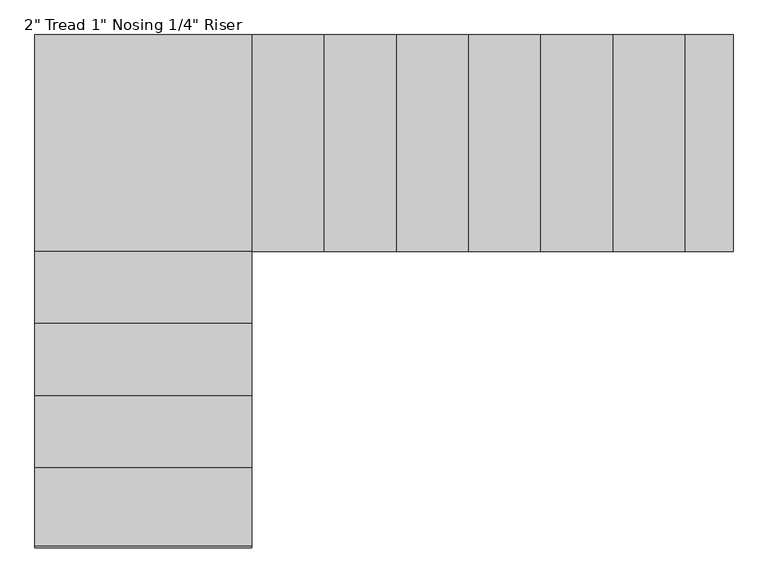
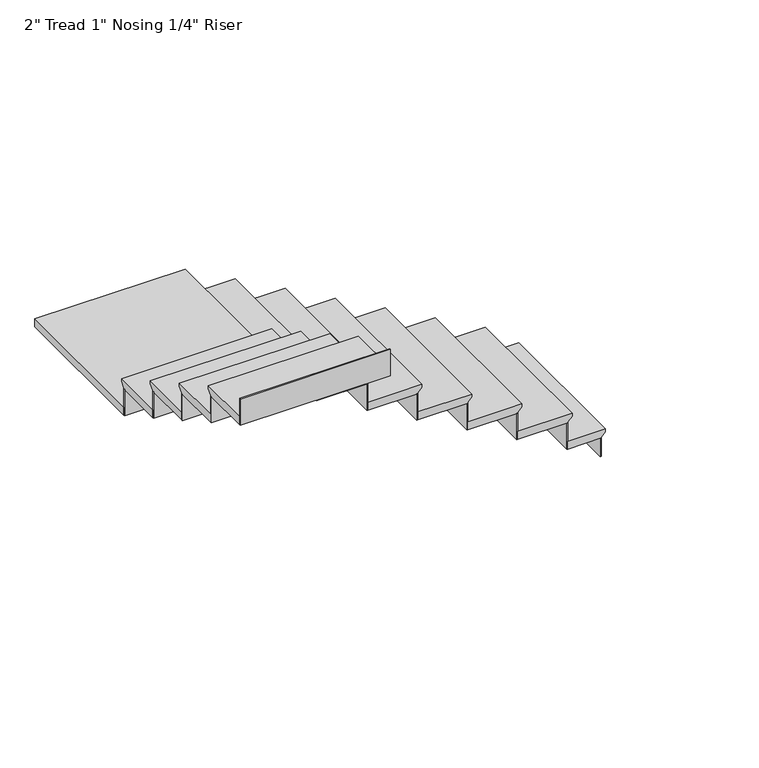
"""IFC4 building model written with IfcOpenShell, lengths in millimetres: stair flight geometry."""

from ifc_helpers import new_model, si_unit, origin, place, context, project, spatial, faceted_brep, source, transform, mapped, element, save


def stair_flight_d8623c0a(model_context):
    return source(origin(), model_context, "Body", "Brep", [
        faceted_brep([(-442.4415084, 5282.3381995, 15999.8833333), (-442.4415084, 5282.3381995, 16018.9333333), (-442.4415084, 4368.3146777, 16018.9333333), (-442.4415084, 4368.3146777, 15999.8833333), (-467.8415084, 5282.3381995, 15974.4833333), (-467.8415084, 4368.3146777, 15974.4833333), (-671.0415084, 5282.3381995, 16018.9333333), (-671.0415084, 4368.3146777, 16018.9333333), (-467.8415084, 4368.3146777, 15968.1333333), (-671.0415084, 4368.3146777, 15968.1333333), (-671.0415084, 5282.3381995, 15968.1333333), (-467.8415084, 5282.3381995, 15968.1333333)], [[[0, 1, 2, 3]], [[4, 0, 3, 5]], [[2, 1, 6, 7]], [[8, 9, 10, 11]], [[2, 7, 9, 8, 5, 3]], [[8, 11, 4, 5]], [[6, 1, 0, 4, 11, 10]], [[7, 6, 10, 9]]]),
        faceted_brep([(-467.8415084, 5282.3381995, 15968.1333333), (-467.8415084, 5282.3381995, 15849.6), (-474.1915084, 5282.3381995, 15849.6), (-474.1915084, 5282.3381995, 15968.1333333), (-467.8415084, 4368.3146777, 15968.1333333), (-474.1915084, 4368.3146777, 15968.1333333), (-474.1915084, 4368.3146777, 15849.6), (-467.8415084, 4368.3146777, 15849.6)], [[[0, 1, 2, 3]], [[4, 5, 6, 7]], [[1, 0, 4, 7]], [[2, 1, 7, 6]], [[3, 2, 6, 5]], [[0, 3, 5, 4]]]),
        faceted_brep([(-671.0415084, 5282.3381995, 16137.4666667), (-671.0415084, 5282.3381995, 15968.1333333), (-677.3915084, 5282.3381995, 15968.1333333), (-677.3915084, 5282.3381995, 16137.4666667), (-671.0415084, 4368.3146777, 16137.4666667), (-677.3915084, 4368.3146777, 16137.4666667), (-677.3915084, 4368.3146777, 15968.1333333), (-671.0415084, 4368.3146777, 15968.1333333)], [[[0, 1, 2, 3]], [[4, 5, 6, 7]], [[1, 0, 4, 7]], [[2, 1, 7, 6]], [[3, 2, 6, 5]], [[0, 3, 5, 4]]]),
        faceted_brep([(-645.6415084, 4368.3146777, 16188.2666667), (-645.6415084, 5282.3381995, 16188.2666667), (-975.8415084, 5282.3381995, 16188.2666667), (-975.8415084, 4368.3146777, 16188.2666667), (-671.0415084, 4368.3146777, 16137.4666667), (-975.8415084, 4368.3146777, 16137.4666667), (-975.8415084, 5282.3381995, 16137.4666667), (-671.0415084, 5282.3381995, 16137.4666667), (-671.0415084, 4368.3146777, 16143.8166667), (-645.6415084, 4368.3146777, 16169.2166667), (-671.0415084, 5282.3381995, 16143.8166667), (-645.6415084, 5282.3381995, 16169.2166667)], [[[0, 1, 2, 3]], [[4, 5, 6, 7]], [[0, 3, 5, 4, 8, 9]], [[4, 7, 10, 8]], [[2, 1, 11, 10, 7, 6]], [[3, 2, 6, 5]], [[11, 1, 0, 9]], [[10, 11, 9, 8]]]),
        faceted_brep([(-975.8415084, 5282.3381995, 16306.8), (-975.8415084, 5282.3381995, 16137.4666667), (-982.1915084, 5282.3381995, 16137.4666667), (-982.1915084, 5282.3381995, 16306.8), (-975.8415084, 4368.3146777, 16306.8), (-982.1915084, 4368.3146777, 16306.8), (-982.1915084, 4368.3146777, 16137.4666667), (-975.8415084, 4368.3146777, 16137.4666667)], [[[0, 1, 2, 3]], [[4, 5, 6, 7]], [[1, 0, 4, 7]], [[2, 1, 7, 6]], [[3, 2, 6, 5]], [[0, 3, 5, 4]]]),
        faceted_brep([(-950.4415084, 4368.3146777, 16357.6), (-950.4415084, 5282.3381995, 16357.6), (-1280.6415084, 5282.3381995, 16357.6), (-1280.6415084, 4368.3146777, 16357.6), (-975.8415084, 4368.3146777, 16306.8), (-1280.6415084, 4368.3146777, 16306.8), (-1280.6415084, 5282.3381995, 16306.8), (-975.8415084, 5282.3381995, 16306.8), (-975.8415084, 4368.3146777, 16313.15), (-950.4415084, 4368.3146777, 16338.55), (-975.8415084, 5282.3381995, 16313.15), (-950.4415084, 5282.3381995, 16338.55)], [[[0, 1, 2, 3]], [[4, 5, 6, 7]], [[0, 3, 5, 4, 8, 9]], [[4, 7, 10, 8]], [[2, 1, 11, 10, 7, 6]], [[3, 2, 6, 5]], [[11, 1, 0, 9]], [[10, 11, 9, 8]]]),
        faceted_brep([(-1280.6415084, 5282.3381995, 16476.1333333), (-1280.6415084, 5282.3381995, 16306.8), (-1286.9915084, 5282.3381995, 16306.8), (-1286.9915084, 5282.3381995, 16476.1333333), (-1280.6415084, 4368.3146777, 16476.1333333), (-1286.9915084, 4368.3146777, 16476.1333333), (-1286.9915084, 4368.3146777, 16306.8), (-1280.6415084, 4368.3146777, 16306.8)], [[[0, 1, 2, 3]], [[4, 5, 6, 7]], [[1, 0, 4, 7]], [[2, 1, 7, 6]], [[3, 2, 6, 5]], [[0, 3, 5, 4]]]),
        faceted_brep([(-1255.2415084, 4368.3146777, 16526.9333333), (-1255.2415084, 5282.3381995, 16526.9333333), (-1585.4415084, 5282.3381995, 16526.9333333), (-1585.4415084, 4368.3146777, 16526.9333333), (-1280.6415084, 4368.3146777, 16476.1333333), (-1585.4415084, 4368.3146777, 16476.1333333), (-1585.4415084, 5282.3381995, 16476.1333333), (-1280.6415084, 5282.3381995, 16476.1333333), (-1280.6415084, 4368.3146777, 16482.4833333), (-1255.2415084, 4368.3146777, 16507.8833333), (-1280.6415084, 5282.3381995, 16482.4833333), (-1255.2415084, 5282.3381995, 16507.8833333)], [[[0, 1, 2, 3]], [[4, 5, 6, 7]], [[0, 3, 5, 4, 8, 9]], [[4, 7, 10, 8]], [[2, 1, 11, 10, 7, 6]], [[3, 2, 6, 5]], [[11, 1, 0, 9]], [[10, 11, 9, 8]]]),
        faceted_brep([(-1585.4415084, 5282.3381995, 16645.4666667), (-1585.4415084, 5282.3381995, 16476.1333333), (-1591.7915084, 5282.3381995, 16476.1333333), (-1591.7915084, 5282.3381995, 16645.4666667), (-1585.4415084, 4368.3146777, 16645.4666667), (-1591.7915084, 4368.3146777, 16645.4666667), (-1591.7915084, 4368.3146777, 16476.1333333), (-1585.4415084, 4368.3146777, 16476.1333333)], [[[0, 1, 2, 3]], [[4, 5, 6, 7]], [[1, 0, 4, 7]], [[2, 1, 7, 6]], [[3, 2, 6, 5]], [[0, 3, 5, 4]]]),
        faceted_brep([(-1560.0415084, 4368.3146777, 16696.2666667), (-1560.0415084, 5282.3381995, 16696.2666667), (-1890.2415084, 5282.3381995, 16696.2666667), (-1890.2415084, 4368.3146777, 16696.2666667), (-1585.4415084, 4368.3146777, 16645.4666667), (-1890.2415084, 4368.3146777, 16645.4666667), (-1890.2415084, 5282.3381995, 16645.4666667), (-1585.4415084, 5282.3381995, 16645.4666667), (-1585.4415084, 4368.3146777, 16651.8166667), (-1560.0415084, 4368.3146777, 16677.2166667), (-1585.4415084, 5282.3381995, 16651.8166667), (-1560.0415084, 5282.3381995, 16677.2166667)], [[[0, 1, 2, 3]], [[4, 5, 6, 7]], [[0, 3, 5, 4, 8, 9]], [[4, 7, 10, 8]], [[2, 1, 11, 10, 7, 6]], [[3, 2, 6, 5]], [[11, 1, 0, 9]], [[10, 11, 9, 8]]]),
        faceted_brep([(-1890.2415084, 5282.3381995, 16814.8), (-1890.2415084, 5282.3381995, 16645.4666667), (-1896.5915084, 5282.3381995, 16645.4666667), (-1896.5915084, 5282.3381995, 16814.8), (-1890.2415084, 4368.3146777, 16814.8), (-1896.5915084, 4368.3146777, 16814.8), (-1896.5915084, 4368.3146777, 16645.4666667), (-1890.2415084, 4368.3146777, 16645.4666667)], [[[0, 1, 2, 3]], [[4, 5, 6, 7]], [[1, 0, 4, 7]], [[2, 1, 7, 6]], [[3, 2, 6, 5]], [[0, 3, 5, 4]]]),
        faceted_brep([(-1864.8415084, 4368.3146777, 16865.6), (-1864.8415084, 5282.3381995, 16865.6), (-2195.0415084, 5282.3381995, 16865.6), (-2195.0415084, 4368.3146777, 16865.6), (-1890.2415084, 4368.3146777, 16814.8), (-2195.0415084, 4368.3146777, 16814.8), (-2195.0415084, 5282.3381995, 16814.8), (-1890.2415084, 5282.3381995, 16814.8), (-1890.2415084, 4368.3146777, 16821.15), (-1864.8415084, 4368.3146777, 16846.55), (-1890.2415084, 5282.3381995, 16821.15), (-1864.8415084, 5282.3381995, 16846.55)], [[[0, 1, 2, 3]], [[4, 5, 6, 7]], [[0, 3, 5, 4, 8, 9]], [[4, 7, 10, 8]], [[2, 1, 11, 10, 7, 6]], [[3, 2, 6, 5]], [[11, 1, 0, 9]], [[10, 11, 9, 8]]]),
        faceted_brep([(-2195.0415084, 5282.3381995, 16984.1333333), (-2195.0415084, 5282.3381995, 16814.8), (-2201.3915084, 5282.3381995, 16814.8), (-2201.3915084, 5282.3381995, 16984.1333333), (-2195.0415084, 4368.3146777, 16984.1333333), (-2201.3915084, 4368.3146777, 16984.1333333), (-2201.3915084, 4368.3146777, 16814.8), (-2195.0415084, 4368.3146777, 16814.8)], [[[0, 1, 2, 3]], [[4, 5, 6, 7]], [[1, 0, 4, 7]], [[2, 1, 7, 6]], [[3, 2, 6, 5]], [[0, 3, 5, 4]]]),
        faceted_brep([(-2169.6415084, 4368.3146777, 17034.9333333), (-2169.6415084, 5282.3381995, 17034.9333333), (-2499.8415084, 5282.3381995, 17034.9333333), (-2499.8415084, 4368.3146777, 17034.9333333), (-2195.0415084, 4368.3146777, 16984.1333333), (-2499.8415084, 4368.3146777, 16984.1333333), (-2499.8415084, 5282.3381995, 16984.1333333), (-2195.0415084, 5282.3381995, 16984.1333333), (-2195.0415084, 4368.3146777, 16990.4833333), (-2169.6415084, 4368.3146777, 17015.8833333), (-2195.0415084, 5282.3381995, 16990.4833333), (-2169.6415084, 5282.3381995, 17015.8833333)], [[[0, 1, 2, 3]], [[4, 5, 6, 7]], [[0, 3, 5, 4, 8, 9]], [[4, 7, 10, 8]], [[2, 1, 11, 10, 7, 6]], [[3, 2, 6, 5]], [[11, 1, 0, 9]], [[10, 11, 9, 8]]]),
        faceted_brep([(-2499.8415084, 5282.3381995, 17153.4666667), (-2499.8415084, 5282.3381995, 16984.1333333), (-2506.1915084, 5282.3381995, 16984.1333333), (-2506.1915084, 5282.3381995, 17153.4666667), (-2499.8415084, 4368.3146777, 17153.4666667), (-2506.1915084, 4368.3146777, 17153.4666667), (-2506.1915084, 4368.3146777, 16984.1333333), (-2499.8415084, 4368.3146777, 16984.1333333)], [[[0, 1, 2, 3]], [[4, 5, 6, 7]], [[1, 0, 4, 7]], [[2, 1, 7, 6]], [[3, 2, 6, 5]], [[0, 3, 5, 4]]]),
        faceted_brep([(-3388.8415084, 5282.3381995, 17204.2666667), (-3388.8415084, 4342.9146777, 17204.2666667), (-2474.4415084, 4342.9146777, 17204.2666667), (-2474.4415084, 5282.3381995, 17204.2666667), (-2474.4415084, 4368.3146777, 17153.4666667), (-2474.4415084, 4342.9146777, 17153.4666667), (-3388.8415084, 4342.9146777, 17153.4666667), (-3388.8415084, 5282.3381995, 17153.4666667), (-2499.8415084, 5282.3381995, 17153.4666667), (-2499.8415084, 4368.3146777, 17153.4666667), (-2474.4415084, 4368.3146777, 17185.2166667), (-2474.4415084, 5282.3381995, 17185.2166667), (-2499.8415084, 4368.3146777, 17159.8166667), (-2499.8415084, 5282.3381995, 17159.8166667)], [[[0, 1, 2, 3]], [[4, 5, 6, 7, 8, 9]], [[3, 2, 5, 4, 10, 11]], [[4, 9, 12, 10]], [[9, 8, 13, 12]], [[0, 3, 11, 13, 8, 7]], [[1, 0, 7, 6]], [[2, 1, 6, 5]], [[13, 11, 10, 12]]]),
        faceted_brep([(-3388.8415084, 4342.9146777, 17322.8), (-3388.8415084, 4342.9146777, 17153.4666667), (-3388.8415084, 4336.5646777, 17153.4666667), (-3388.8415084, 4336.5646777, 17322.8), (-2474.4415084, 4342.9146777, 17322.8), (-2474.4415084, 4336.5646777, 17322.8), (-2474.4415084, 4336.5646777, 17153.4666667), (-2474.4415084, 4342.9146777, 17153.4666667)], [[[0, 1, 2, 3]], [[4, 5, 6, 7]], [[1, 0, 4, 7]], [[2, 1, 7, 6]], [[3, 2, 6, 5]], [[0, 3, 5, 4]]]),
        faceted_brep([(-2474.4415084, 4368.3146777, 17373.6), (-3388.8415084, 4368.3146777, 17373.6), (-3388.8415084, 4037.7382512, 17373.6), (-2474.4415084, 4037.7382512, 17373.6), (-2474.4415084, 4342.9146777, 17322.8), (-2474.4415084, 4037.7382512, 17322.8), (-3388.8415084, 4037.7382512, 17322.8), (-3388.8415084, 4342.9146777, 17322.8), (-2474.4415084, 4342.9146777, 17329.15), (-2474.4415084, 4368.3146777, 17354.55), (-3388.8415084, 4342.9146777, 17329.15), (-3388.8415084, 4368.3146777, 17354.55)], [[[0, 1, 2, 3]], [[4, 5, 6, 7]], [[0, 3, 5, 4, 8, 9]], [[4, 7, 10, 8]], [[2, 1, 11, 10, 7, 6]], [[3, 2, 6, 5]], [[11, 1, 0, 9]], [[10, 11, 9, 8]]]),
        faceted_brep([(-3388.8415084, 4037.7382512, 17492.1333333), (-3388.8415084, 4037.7382512, 17322.8), (-3388.8415084, 4031.3882512, 17322.8), (-3388.8415084, 4031.3882512, 17492.1333333), (-2474.4415084, 4037.7382512, 17492.1333333), (-2474.4415084, 4031.3882512, 17492.1333333), (-2474.4415084, 4031.3882512, 17322.8), (-2474.4415084, 4037.7382512, 17322.8)], [[[0, 1, 2, 3]], [[4, 5, 6, 7]], [[1, 0, 4, 7]], [[2, 1, 7, 6]], [[3, 2, 6, 5]], [[0, 3, 5, 4]]]),
        faceted_brep([(-2474.4415084, 4063.1382512, 17542.9333333), (-3388.8415084, 4063.1382512, 17542.9333333), (-3388.8415084, 3732.938277, 17542.9333333), (-2474.4415084, 3732.938277, 17542.9333333), (-2474.4415084, 4037.7382512, 17492.1333333), (-2474.4415084, 3732.938277, 17492.1333333), (-3388.8415084, 3732.938277, 17492.1333333), (-3388.8415084, 4037.7382512, 17492.1333333), (-2474.4415084, 4037.7382512, 17498.4833333), (-2474.4415084, 4063.1382512, 17523.8833333), (-3388.8415084, 4037.7382512, 17498.4833333), (-3388.8415084, 4063.1382512, 17523.8833333)], [[[0, 1, 2, 3]], [[4, 5, 6, 7]], [[0, 3, 5, 4, 8, 9]], [[4, 7, 10, 8]], [[2, 1, 11, 10, 7, 6]], [[3, 2, 6, 5]], [[11, 1, 0, 9]], [[10, 11, 9, 8]]]),
        faceted_brep([(-3388.8415084, 3732.938277, 17661.4666667), (-3388.8415084, 3732.938277, 17492.1333333), (-3388.8415084, 3726.588277, 17492.1333333), (-3388.8415084, 3726.588277, 17661.4666667), (-2474.4415084, 3732.938277, 17661.4666667), (-2474.4415084, 3726.588277, 17661.4666667), (-2474.4415084, 3726.588277, 17492.1333333), (-2474.4415084, 3732.938277, 17492.1333333)], [[[0, 1, 2, 3]], [[4, 5, 6, 7]], [[1, 0, 4, 7]], [[2, 1, 7, 6]], [[3, 2, 6, 5]], [[0, 3, 5, 4]]]),
        faceted_brep([(-2474.4415084, 3758.338277, 17712.2666667), (-3388.8415084, 3758.338277, 17712.2666667), (-3388.8415084, 3428.1383028, 17712.2666667), (-2474.4415084, 3428.1383028, 17712.2666667), (-2474.4415084, 3732.938277, 17661.4666667), (-2474.4415084, 3428.1383028, 17661.4666667), (-3388.8415084, 3428.1383028, 17661.4666667), (-3388.8415084, 3732.938277, 17661.4666667), (-2474.4415084, 3732.938277, 17667.8166667), (-2474.4415084, 3758.338277, 17693.2166667), (-3388.8415084, 3732.938277, 17667.8166667), (-3388.8415084, 3758.338277, 17693.2166667)], [[[0, 1, 2, 3]], [[4, 5, 6, 7]], [[0, 3, 5, 4, 8, 9]], [[4, 7, 10, 8]], [[2, 1, 11, 10, 7, 6]], [[3, 2, 6, 5]], [[11, 1, 0, 9]], [[10, 11, 9, 8]]]),
        faceted_brep([(-3388.8415084, 3428.1383028, 17830.8), (-3388.8415084, 3428.1383028, 17661.4666667), (-3388.8415084, 3421.7883028, 17661.4666667), (-3388.8415084, 3421.7883028, 17830.8), (-2474.4415084, 3428.1383028, 17830.8), (-2474.4415084, 3421.7883028, 17830.8), (-2474.4415084, 3421.7883028, 17661.4666667), (-2474.4415084, 3428.1383028, 17661.4666667)], [[[0, 1, 2, 3]], [[4, 5, 6, 7]], [[1, 0, 4, 7]], [[2, 1, 7, 6]], [[3, 2, 6, 5]], [[0, 3, 5, 4]]]),
        faceted_brep([(-3388.8415084, 3123.3383287, 18000.1333333), (-3388.8415084, 3123.3383287, 17830.8), (-3388.8415084, 3116.9883287, 17830.8), (-3388.8415084, 3116.9883287, 18000.1333333), (-2474.4415084, 3123.3383287, 18000.1333333), (-2474.4415084, 3116.9883287, 18000.1333333), (-2474.4415084, 3116.9883287, 17830.8), (-2474.4415084, 3123.3383287, 17830.8)], [[[0, 1, 2, 3]], [[4, 5, 6, 7]], [[1, 0, 4, 7]], [[2, 1, 7, 6]], [[3, 2, 6, 5]], [[0, 3, 5, 4]]]),
        faceted_brep([(-2474.4415084, 3453.5383028, 17881.6), (-3388.8415084, 3453.5383028, 17881.6), (-3388.8415084, 3123.3383287, 17881.6), (-2474.4415084, 3123.3383287, 17881.6), (-2474.4415084, 3428.1383028, 17830.8), (-2474.4415084, 3123.3383287, 17830.8), (-3388.8415084, 3123.3383287, 17830.8), (-3388.8415084, 3428.1383028, 17830.8), (-2474.4415084, 3428.1383028, 17837.15), (-2474.4415084, 3453.5383028, 17862.55), (-3388.8415084, 3428.1383028, 17837.15), (-3388.8415084, 3453.5383028, 17862.55)], [[[0, 1, 2, 3]], [[4, 5, 6, 7]], [[0, 3, 5, 4, 8, 9]], [[4, 7, 10, 8]], [[2, 1, 11, 10, 7, 6]], [[3, 2, 6, 5]], [[11, 1, 0, 9]], [[10, 11, 9, 8]]]),
    ])


if __name__ == "__main__":
    model = new_model("IFC4")
    model_context = context("Model", 3, world=origin())
    ifc_project = project(units=[si_unit("LENGTHUNIT", "METRE", prefix="MILLI")], contexts=[model_context])
    site = spatial("IfcSite", under=ifc_project)
    building = spatial("IfcBuilding", under=site)
    placement = place(None, origin())
    stair_flight_shape = stair_flight_d8623c0a(model_context)
    element("IfcStairFlight", 1, ObjectType="2\" Tread 1\" Nosing 1/4\" Riser", at=placement, inside=building, context=model_context, shape_type="MappedRepresentation", body=[
        mapped(stair_flight_shape, transform((0.0, 0.0, 0.0), x_axis=(1.0, 0.0, 0.0), y_axis=(0.0, 1.0, 0.0), z_axis=(0.0, 0.0, 1.0))),
    ])
    save(model, "model.ifc")
